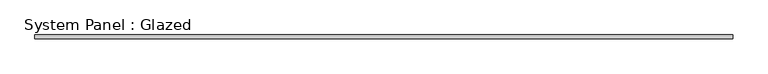
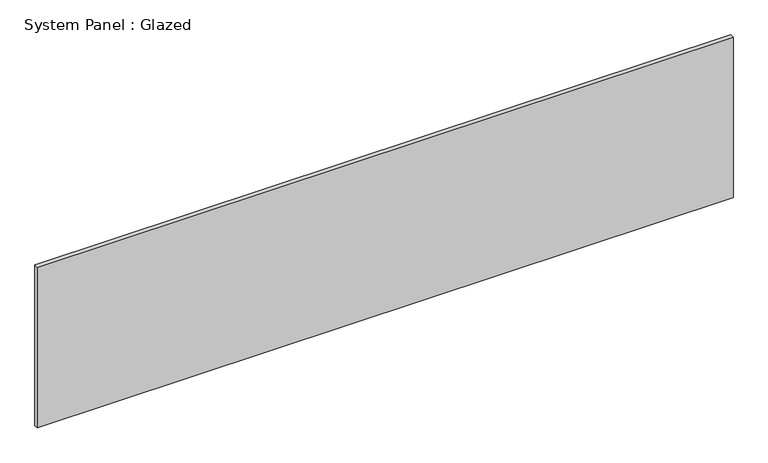
"""IFC4 building model written with IfcOpenShell, lengths in millimetres: plate geometry, System Panel : Glazed."""

from ifc_helpers import new_model, si_unit, origin, origin_with_axes, place, context, project, spatial, polyline, outline, extrude, source, transform, mapped, element, save


def system_panel_glazed_64dbbd21(model_context):
    return source(origin(), model_context, "Body", "SweptSolid", [
        extrude(outline(polyline([(2368.1420746, 19.05), (-2368.1420746, 19.05), (-2368.1420746, 44.45), (2368.1420746, 44.45), (2368.1420746, 19.05)])), origin_with_axes(), (0.0, 0.0, 1.0), 1155.7),
    ])


if __name__ == "__main__":
    model = new_model("IFC4")
    model_context = context("Model", 3, world=origin())
    ifc_project = project(units=[si_unit("LENGTHUNIT", "METRE", prefix="MILLI")], contexts=[model_context])
    site = spatial("IfcSite", under=ifc_project)
    building = spatial("IfcBuilding", under=site)
    placement = place(None, origin())
    system_panel_glazed_shape = system_panel_glazed_64dbbd21(model_context)
    element("IfcPlate", 1, ObjectType="System Panel : Glazed", at=placement, inside=building, context=model_context, shape_type="MappedRepresentation", body=[
        mapped(system_panel_glazed_shape, transform((0.0, 0.0, 0.0), x_axis=(1.0, 0.0, 0.0), y_axis=(0.0, 1.0, 0.0), z_axis=(0.0, 0.0, 1.0))),
    ])
    save(model, "model.ifc")

# Revit data of these elements
# Type "System Panel : Glazed"
#   Construction Type Id = "GSP4R"
#   Analytic Construction = "1/8 in Pilkington single glazing"
#   Visual Light Transmittance = 0.9
#   Solar Heat Gain Coefficient = 0.86
#   Heat Transfer Coefficient (U) = 1.18115 BTU/(h·ft²·°F)
# Element 1 (IfcPlate, "System Panel : Glazed")
#   Materials on its faces: "Glass"
# Materials
#   "Glass": class "Glass", colour RGB 0 128 192, transparency 0.75, Description = "Soda Lime Glass", Cost = 0
